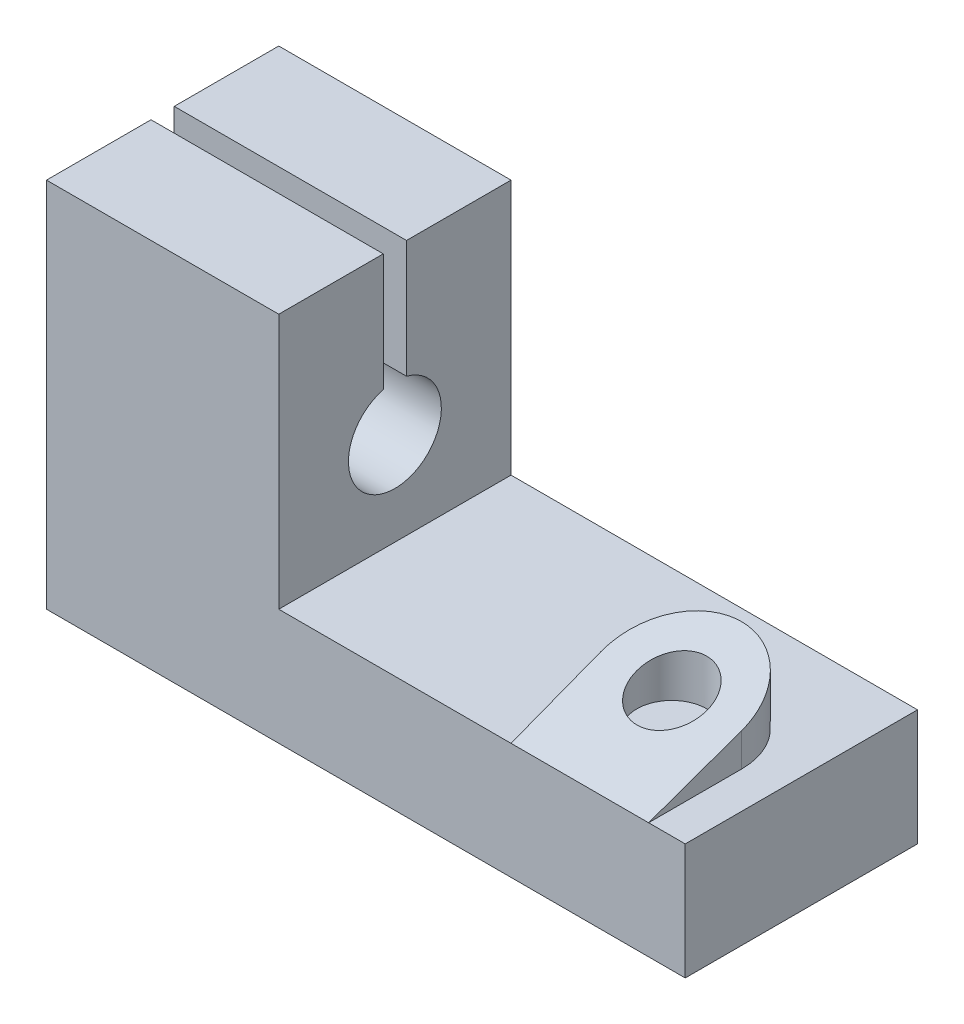
ISO-10303-21;
HEADER;
FILE_DESCRIPTION(('STEP AP214'),'2;1');
FILE_NAME('part.step','',(''),(''),'','','');
FILE_SCHEMA(('AUTOMOTIVE_DESIGN { 1 0 10303 214 1 1 1 1 }'));
ENDSEC;
DATA;
#1=APPLICATION_CONTEXT('core data for automotive mechanical design processes');
#2=APPLICATION_PROTOCOL_DEFINITION('international standard','automotive_design',2000,#1);
#3=PRODUCT_CONTEXT('',#1,'mechanical');
#4=PRODUCT('Part','Part','',(#3));
#5=PRODUCT_RELATED_PRODUCT_CATEGORY('part','',(#4));
#6=PRODUCT_DEFINITION_FORMATION('','',#4);
#7=PRODUCT_DEFINITION_CONTEXT('part definition',#1,'design');
#8=PRODUCT_DEFINITION('design','',#6,#7);
#9=PRODUCT_DEFINITION_SHAPE('','',#8);
#10=(LENGTH_UNIT() NAMED_UNIT(*) SI_UNIT(.MILLI.,.METRE.));
#11=(NAMED_UNIT(*) PLANE_ANGLE_UNIT() SI_UNIT($,.RADIAN.));
#12=(NAMED_UNIT(*) SI_UNIT($,.STERADIAN.) SOLID_ANGLE_UNIT());
#13=UNCERTAINTY_MEASURE_WITH_UNIT(LENGTH_MEASURE(1.E-05),#10,'distance_accuracy_value','');
#14=(GEOMETRIC_REPRESENTATION_CONTEXT(3) GLOBAL_UNCERTAINTY_ASSIGNED_CONTEXT((#13)) GLOBAL_UNIT_ASSIGNED_CONTEXT((#10,
#11,#12)) REPRESENTATION_CONTEXT('',''));
#15=CARTESIAN_POINT('',(0.,0.,0.));
#16=DIRECTION('',(0.,0.,1.));
#17=DIRECTION('',(1.,0.,0.));
#18=AXIS2_PLACEMENT_3D('',#15,#16,#17);
#19=CARTESIAN_POINT('',(0.,0.,20.));
#20=DIRECTION('',(1.,0.,0.));
#21=DIRECTION('',(0.,0.,-1.));
#22=AXIS2_PLACEMENT_3D('',#19,#20,#21);
#23=PLANE('',#22);
#24=DIRECTION('',(0.,1.,0.));
#25=VECTOR('',#24,1.);
#26=CARTESIAN_POINT('',(0.,0.,11.));
#27=LINE('',#26,#25);
#28=CARTESIAN_POINT('',(0.,21.8729833462074,11.));
#29=VERTEX_POINT('',#28);
#30=CARTESIAN_POINT('',(0.,32.,11.));
#31=VERTEX_POINT('',#30);
#32=EDGE_CURVE('E162',#29,#31,#27,.T.);
#33=ORIENTED_EDGE('',*,*,#32,.F.);
#34=CARTESIAN_POINT('',(0.,18.,10.));
#35=DIRECTION('',(1.,0.,0.));
#36=DIRECTION('',(0.,0.,-1.));
#37=AXIS2_PLACEMENT_3D('',#34,#35,#36);
#38=CIRCLE('',#37,4.);
#39=CARTESIAN_POINT('',(0.,21.8729833462074,9.));
#40=VERTEX_POINT('',#39);
#41=EDGE_CURVE('E176',#29,#40,#38,.T.);
#42=ORIENTED_EDGE('',*,*,#41,.T.);
#43=DIRECTION('',(0.,1.,0.));
#44=VECTOR('',#43,1.);
#45=CARTESIAN_POINT('',(0.,0.,9.));
#46=LINE('',#45,#44);
#47=CARTESIAN_POINT('',(0.,32.,9.));
#48=VERTEX_POINT('',#47);
#49=EDGE_CURVE('E64',#40,#48,#46,.T.);
#50=ORIENTED_EDGE('',*,*,#49,.T.);
#51=DIRECTION('',(0.,0.,-1.));
#52=VECTOR('',#51,1.);
#53=CARTESIAN_POINT('',(0.,32.,20.));
#54=LINE('',#53,#52);
#55=CARTESIAN_POINT('',(0.,32.,0.));
#56=VERTEX_POINT('',#55);
#57=EDGE_CURVE('E203',#48,#56,#54,.T.);
#58=ORIENTED_EDGE('',*,*,#57,.T.);
#59=DIRECTION('',(0.,-1.,0.));
#60=VECTOR('',#59,1.);
#61=CARTESIAN_POINT('',(0.,0.,0.));
#62=LINE('',#61,#60);
#63=CARTESIAN_POINT('',(0.,0.,0.));
#64=VERTEX_POINT('',#63);
#65=EDGE_CURVE('E185',#56,#64,#62,.T.);
#66=ORIENTED_EDGE('',*,*,#65,.T.);
#67=DIRECTION('',(0.,0.,-1.));
#68=VECTOR('',#67,1.);
#69=CARTESIAN_POINT('',(0.,0.,20.));
#70=LINE('',#69,#68);
#71=CARTESIAN_POINT('',(0.,0.,20.));
#72=VERTEX_POINT('',#71);
#73=EDGE_CURVE('E11',#72,#64,#70,.T.);
#74=ORIENTED_EDGE('',*,*,#73,.F.);
#75=DIRECTION('',(0.,-1.,0.));
#76=VECTOR('',#75,1.);
#77=CARTESIAN_POINT('',(0.,0.,20.));
#78=LINE('',#77,#76);
#79=CARTESIAN_POINT('',(0.,32.,20.));
#80=VERTEX_POINT('',#79);
#81=EDGE_CURVE('E183',#80,#72,#78,.T.);
#82=ORIENTED_EDGE('',*,*,#81,.F.);
#83=EDGE_CURVE('E214',#80,#31,#54,.T.);
#84=ORIENTED_EDGE('',*,*,#83,.T.);
#85=EDGE_LOOP('',(#33,#42,#50,#58,#66,#74,#82,#84));
#86=FACE_BOUND('',#85,.T.);
#87=ADVANCED_FACE('F39',(#86),#23,.F.);
#88=CARTESIAN_POINT('',(20.,32.,20.));
#89=DIRECTION('',(-1.,0.,0.));
#90=DIRECTION('',(0.,0.,1.));
#91=AXIS2_PLACEMENT_3D('',#88,#89,#90);
#92=PLANE('',#91);
#93=DIRECTION('',(0.,1.,0.));
#94=VECTOR('',#93,1.);
#95=CARTESIAN_POINT('',(20.,0.,11.));
#96=LINE('',#95,#94);
#97=CARTESIAN_POINT('',(20.,21.8729833462074,11.));
#98=VERTEX_POINT('',#97);
#99=CARTESIAN_POINT('',(20.,32.,11.));
#100=VERTEX_POINT('',#99);
#101=EDGE_CURVE('E53',#98,#100,#96,.T.);
#102=ORIENTED_EDGE('',*,*,#101,.T.);
#103=DIRECTION('',(0.,0.,-1.));
#104=VECTOR('',#103,1.);
#105=CARTESIAN_POINT('',(20.,32.,20.));
#106=LINE('',#105,#104);
#107=CARTESIAN_POINT('',(20.,32.,20.));
#108=VERTEX_POINT('',#107);
#109=EDGE_CURVE('E218',#108,#100,#106,.T.);
#110=ORIENTED_EDGE('',*,*,#109,.F.);
#111=DIRECTION('',(0.,1.,0.));
#112=VECTOR('',#111,1.);
#113=CARTESIAN_POINT('',(20.,32.,20.));
#114=LINE('',#113,#112);
#115=CARTESIAN_POINT('',(20.,10.,20.));
#116=VERTEX_POINT('',#115);
#117=EDGE_CURVE('E197',#116,#108,#114,.T.);
#118=ORIENTED_EDGE('',*,*,#117,.F.);
#119=DIRECTION('',(0.,0.,-1.));
#120=VECTOR('',#119,1.);
#121=CARTESIAN_POINT('',(20.,10.,20.));
#122=LINE('',#121,#120);
#123=CARTESIAN_POINT('',(20.,10.,0.));
#124=VERTEX_POINT('',#123);
#125=EDGE_CURVE('E225',#116,#124,#122,.T.);
#126=ORIENTED_EDGE('',*,*,#125,.T.);
#127=DIRECTION('',(0.,1.,0.));
#128=VECTOR('',#127,1.);
#129=CARTESIAN_POINT('',(20.,32.,0.));
#130=LINE('',#129,#128);
#131=CARTESIAN_POINT('',(20.,32.,0.));
#132=VERTEX_POINT('',#131);
#133=EDGE_CURVE('E209',#124,#132,#130,.T.);
#134=ORIENTED_EDGE('',*,*,#133,.T.);
#135=CARTESIAN_POINT('',(20.,32.,9.));
#136=VERTEX_POINT('',#135);
#137=EDGE_CURVE('E217',#136,#132,#106,.T.);
#138=ORIENTED_EDGE('',*,*,#137,.F.);
#139=DIRECTION('',(0.,1.,0.));
#140=VECTOR('',#139,1.);
#141=CARTESIAN_POINT('',(20.,0.,9.));
#142=LINE('',#141,#140);
#143=CARTESIAN_POINT('',(20.,21.8729833462074,9.));
#144=VERTEX_POINT('',#143);
#145=EDGE_CURVE('E164',#144,#136,#142,.T.);
#146=ORIENTED_EDGE('',*,*,#145,.F.);
#147=CARTESIAN_POINT('',(20.,18.,10.));
#148=DIRECTION('',(1.,0.,0.));
#149=DIRECTION('',(0.,0.,-1.));
#150=AXIS2_PLACEMENT_3D('',#147,#148,#149);
#151=CIRCLE('',#150,4.);
#152=EDGE_CURVE('E174',#98,#144,#151,.T.);
#153=ORIENTED_EDGE('',*,*,#152,.F.);
#154=EDGE_LOOP('',(#102,#110,#118,#126,#134,#138,#146,#153));
#155=FACE_BOUND('',#154,.T.);
#156=ADVANCED_FACE('F248',(#155),#92,.F.);
#157=CARTESIAN_POINT('',(0.,32.,20.));
#158=DIRECTION('',(0.,-1.,0.));
#159=DIRECTION('',(0.,0.,-1.));
#160=AXIS2_PLACEMENT_3D('',#157,#158,#159);
#161=PLANE('',#160);
#162=DIRECTION('',(1.,0.,0.));
#163=VECTOR('',#162,1.);
#164=CARTESIAN_POINT('',(0.,32.,11.));
#165=LINE('',#164,#163);
#166=EDGE_CURVE('E168',#31,#100,#165,.T.);
#167=ORIENTED_EDGE('',*,*,#166,.F.);
#168=ORIENTED_EDGE('',*,*,#83,.F.);
#169=DIRECTION('',(-1.,0.,0.));
#170=VECTOR('',#169,1.);
#171=CARTESIAN_POINT('',(0.,32.,20.));
#172=LINE('',#171,#170);
#173=EDGE_CURVE('E200',#108,#80,#172,.T.);
#174=ORIENTED_EDGE('',*,*,#173,.F.);
#175=ORIENTED_EDGE('',*,*,#109,.T.);
#176=EDGE_LOOP('',(#167,#168,#174,#175));
#177=FACE_BOUND('',#176,.T.);
#178=ADVANCED_FACE('F291',(#177),#161,.F.);
#179=CARTESIAN_POINT('',(0.,18.,10.));
#180=DIRECTION('',(1.,0.,0.));
#181=DIRECTION('',(0.,0.,-1.));
#182=AXIS2_PLACEMENT_3D('',#179,#180,#181);
#183=CYLINDRICAL_SURFACE('',#182,4.);
#184=DIRECTION('',(1.,0.,0.));
#185=VECTOR('',#184,1.);
#186=CARTESIAN_POINT('',(0.,21.8729833462074,11.));
#187=LINE('',#186,#185);
#188=EDGE_CURVE('E170',#29,#98,#187,.T.);
#189=ORIENTED_EDGE('',*,*,#188,.T.);
#190=ORIENTED_EDGE('',*,*,#152,.T.);
#191=DIRECTION('',(1.,0.,0.));
#192=VECTOR('',#191,1.);
#193=CARTESIAN_POINT('',(0.,21.8729833462074,9.));
#194=LINE('',#193,#192);
#195=EDGE_CURVE('E177',#40,#144,#194,.T.);
#196=ORIENTED_EDGE('',*,*,#195,.F.);
#197=ORIENTED_EDGE('',*,*,#41,.F.);
#198=EDGE_LOOP('',(#189,#190,#196,#197));
#199=FACE_BOUND('',#198,.T.);
#200=ADVANCED_FACE('F296',(#199),#183,.F.);
#201=CARTESIAN_POINT('',(0.,0.,20.));
#202=DIRECTION('',(0.,1.,0.));
#203=DIRECTION('',(0.,0.,1.));
#204=AXIS2_PLACEMENT_3D('',#201,#202,#203);
#205=PLANE('',#204);
#206=DIRECTION('',(1.,0.,0.));
#207=VECTOR('',#206,1.);
#208=CARTESIAN_POINT('',(0.,0.,0.));
#209=LINE('',#208,#207);
#210=CARTESIAN_POINT('',(55.,0.,0.));
#211=VERTEX_POINT('',#210);
#212=EDGE_CURVE('E204',#64,#211,#209,.T.);
#213=ORIENTED_EDGE('',*,*,#212,.T.);
#214=DIRECTION('',(0.,0.,-1.));
#215=VECTOR('',#214,1.);
#216=CARTESIAN_POINT('',(55.,0.,20.));
#217=LINE('',#216,#215);
#218=CARTESIAN_POINT('',(55.,0.,20.));
#219=VERTEX_POINT('',#218);
#220=EDGE_CURVE('E50',#219,#211,#217,.T.);
#221=ORIENTED_EDGE('',*,*,#220,.F.);
#222=DIRECTION('',(1.,0.,0.));
#223=VECTOR('',#222,1.);
#224=CARTESIAN_POINT('',(0.,0.,20.));
#225=LINE('',#224,#223);
#226=EDGE_CURVE('E190',#72,#219,#225,.T.);
#227=ORIENTED_EDGE('',*,*,#226,.F.);
#228=ORIENTED_EDGE('',*,*,#73,.T.);
#229=EDGE_LOOP('',(#213,#221,#227,#228));
#230=FACE_BOUND('',#229,.T.);
#231=ADVANCED_FACE('F308',(#230),#205,.F.);
#232=CARTESIAN_POINT('',(55.,0.,20.));
#233=DIRECTION('',(-1.,0.,0.));
#234=DIRECTION('',(0.,0.,1.));
#235=AXIS2_PLACEMENT_3D('',#232,#233,#234);
#236=PLANE('',#235);
#237=DIRECTION('',(0.,1.,0.));
#238=VECTOR('',#237,1.);
#239=CARTESIAN_POINT('',(55.,0.,0.));
#240=LINE('',#239,#238);
#241=CARTESIAN_POINT('',(55.,10.,0.));
#242=VERTEX_POINT('',#241);
#243=EDGE_CURVE('E206',#211,#242,#240,.T.);
#244=ORIENTED_EDGE('',*,*,#243,.T.);
#245=DIRECTION('',(0.,0.,-1.));
#246=VECTOR('',#245,1.);
#247=CARTESIAN_POINT('',(55.,10.,20.));
#248=LINE('',#247,#246);
#249=CARTESIAN_POINT('',(55.,10.,20.));
#250=VERTEX_POINT('',#249);
#251=EDGE_CURVE('E223',#250,#242,#248,.T.);
#252=ORIENTED_EDGE('',*,*,#251,.F.);
#253=DIRECTION('',(0.,1.,0.));
#254=VECTOR('',#253,1.);
#255=CARTESIAN_POINT('',(55.,0.,20.));
#256=LINE('',#255,#254);
#257=EDGE_CURVE('E192',#219,#250,#256,.T.);
#258=ORIENTED_EDGE('',*,*,#257,.F.);
#259=ORIENTED_EDGE('',*,*,#220,.T.);
#260=EDGE_LOOP('',(#244,#252,#258,#259));
#261=FACE_BOUND('',#260,.T.);
#262=ADVANCED_FACE('F235',(#261),#236,.F.);
#263=CARTESIAN_POINT('',(20.,10.,20.));
#264=DIRECTION('',(0.,-1.,0.));
#265=DIRECTION('',(0.,0.,-1.));
#266=AXIS2_PLACEMENT_3D('',#263,#264,#265);
#267=PLANE('',#266);
#268=DIRECTION('',(0.0193826635216767,0.,0.999812138531437));
#269=VECTOR('',#268,1.);
#270=CARTESIAN_POINT('',(39.8471641057222,10.,12.1162959811301));
#271=LINE('',#270,#269);
#272=CARTESIAN_POINT('',(39.8471641057222,10.,12.1162959811301));
#273=VERTEX_POINT('',#272);
#274=CARTESIAN_POINT('',(40.,10.,20.));
#275=VERTEX_POINT('',#274);
#276=EDGE_CURVE('E157',#273,#275,#271,.T.);
#277=ORIENTED_EDGE('',*,*,#276,.F.);
#278=CARTESIAN_POINT('',(45.8460369369108,10.,12.));
#279=DIRECTION('',(0.,1.,0.));
#280=DIRECTION('',(0.,0.,1.));
#281=AXIS2_PLACEMENT_3D('',#278,#279,#280);
#282=CIRCLE('',#281,6.);
#283=CARTESIAN_POINT('',(51.8460369369108,10.,12.));
#284=VERTEX_POINT('',#283);
#285=EDGE_CURVE('E256',#284,#273,#282,.T.);
#286=ORIENTED_EDGE('',*,*,#285,.F.);
#287=DIRECTION('',(0.,0.,-1.));
#288=VECTOR('',#287,1.);
#289=CARTESIAN_POINT('',(51.8460369369108,10.,20.));
#290=LINE('',#289,#288);
#291=CARTESIAN_POINT('',(51.8460369369108,10.,20.));
#292=VERTEX_POINT('',#291);
#293=EDGE_CURVE('E154',#292,#284,#290,.T.);
#294=ORIENTED_EDGE('',*,*,#293,.F.);
#295=DIRECTION('',(-1.,0.,0.));
#296=VECTOR('',#295,1.);
#297=CARTESIAN_POINT('',(20.,10.,20.));
#298=LINE('',#297,#296);
#299=EDGE_CURVE('E191',#250,#292,#298,.T.);
#300=ORIENTED_EDGE('',*,*,#299,.F.);
#301=ORIENTED_EDGE('',*,*,#251,.T.);
#302=DIRECTION('',(-1.,0.,0.));
#303=VECTOR('',#302,1.);
#304=CARTESIAN_POINT('',(20.,10.,0.));
#305=LINE('',#304,#303);
#306=EDGE_CURVE('E208',#242,#124,#305,.T.);
#307=ORIENTED_EDGE('',*,*,#306,.T.);
#308=ORIENTED_EDGE('',*,*,#125,.F.);
#309=EDGE_CURVE('E195',#275,#116,#298,.T.);
#310=ORIENTED_EDGE('',*,*,#309,.F.);
#311=EDGE_LOOP('',(#277,#286,#294,#300,#301,#307,#308,#310));
#312=FACE_BOUND('',#311,.T.);
#313=ADVANCED_FACE('F243',(#312),#267,.F.);
#314=ORIENTED_EDGE('',*,*,#57,.F.);
#315=DIRECTION('',(1.,0.,0.));
#316=VECTOR('',#315,1.);
#317=CARTESIAN_POINT('',(0.,32.,9.));
#318=LINE('',#317,#316);
#319=EDGE_CURVE('E175',#48,#136,#318,.T.);
#320=ORIENTED_EDGE('',*,*,#319,.T.);
#321=ORIENTED_EDGE('',*,*,#137,.T.);
#322=DIRECTION('',(-1.,0.,0.));
#323=VECTOR('',#322,1.);
#324=CARTESIAN_POINT('',(0.,32.,0.));
#325=LINE('',#324,#323);
#326=EDGE_CURVE('E186',#132,#56,#325,.T.);
#327=ORIENTED_EDGE('',*,*,#326,.T.);
#328=EDGE_LOOP('',(#314,#320,#321,#327));
#329=FACE_BOUND('',#328,.T.);
#330=ADVANCED_FACE('F287',(#329),#161,.F.);
#331=CARTESIAN_POINT('',(0.,0.,20.));
#332=DIRECTION('',(0.,0.,-1.));
#333=DIRECTION('',(-1.,0.,0.));
#334=AXIS2_PLACEMENT_3D('',#331,#332,#333);
#335=PLANE('',#334);
#336=ORIENTED_EDGE('',*,*,#299,.T.);
#337=DIRECTION('',(1.,0.,0.));
#338=VECTOR('',#337,1.);
#339=CARTESIAN_POINT('',(39.8460369369108,10.,20.));
#340=LINE('',#339,#338);
#341=EDGE_CURVE('E147',#275,#292,#340,.T.);
#342=ORIENTED_EDGE('',*,*,#341,.F.);
#343=ORIENTED_EDGE('',*,*,#309,.T.);
#344=ORIENTED_EDGE('',*,*,#117,.T.);
#345=ORIENTED_EDGE('',*,*,#173,.T.);
#346=ORIENTED_EDGE('',*,*,#81,.T.);
#347=ORIENTED_EDGE('',*,*,#226,.T.);
#348=ORIENTED_EDGE('',*,*,#257,.T.);
#349=EDGE_LOOP('',(#336,#342,#343,#344,#345,#346,#347,#348));
#350=FACE_BOUND('',#349,.T.);
#351=ADVANCED_FACE('F254',(#350),#335,.F.);
#352=CARTESIAN_POINT('',(0.,0.,0.));
#353=DIRECTION('',(0.,0.,-1.));
#354=DIRECTION('',(-1.,0.,0.));
#355=AXIS2_PLACEMENT_3D('',#352,#353,#354);
#356=PLANE('',#355);
#357=ORIENTED_EDGE('',*,*,#65,.F.);
#358=ORIENTED_EDGE('',*,*,#326,.F.);
#359=ORIENTED_EDGE('',*,*,#133,.F.);
#360=ORIENTED_EDGE('',*,*,#306,.F.);
#361=ORIENTED_EDGE('',*,*,#243,.F.);
#362=ORIENTED_EDGE('',*,*,#212,.F.);
#363=EDGE_LOOP('',(#357,#358,#359,#360,#361,#362));
#364=FACE_BOUND('',#363,.T.);
#365=ADVANCED_FACE('F239',(#364),#356,.T.);
#366=CARTESIAN_POINT('',(0.,0.,9.));
#367=DIRECTION('',(0.,0.,-1.));
#368=DIRECTION('',(-1.,0.,0.));
#369=AXIS2_PLACEMENT_3D('',#366,#367,#368);
#370=PLANE('',#369);
#371=ORIENTED_EDGE('',*,*,#145,.T.);
#372=ORIENTED_EDGE('',*,*,#319,.F.);
#373=ORIENTED_EDGE('',*,*,#49,.F.);
#374=ORIENTED_EDGE('',*,*,#195,.T.);
#375=EDGE_LOOP('',(#371,#372,#373,#374));
#376=FACE_BOUND('',#375,.T.);
#377=ADVANCED_FACE('F304',(#376),#370,.F.);
#378=CARTESIAN_POINT('',(0.,0.,11.));
#379=DIRECTION('',(0.,0.,-1.));
#380=DIRECTION('',(-1.,0.,0.));
#381=AXIS2_PLACEMENT_3D('',#378,#379,#380);
#382=PLANE('',#381);
#383=ORIENTED_EDGE('',*,*,#101,.F.);
#384=ORIENTED_EDGE('',*,*,#188,.F.);
#385=ORIENTED_EDGE('',*,*,#32,.T.);
#386=ORIENTED_EDGE('',*,*,#166,.T.);
#387=EDGE_LOOP('',(#383,#384,#385,#386));
#388=FACE_BOUND('',#387,.T.);
#389=ADVANCED_FACE('F321',(#388),#382,.T.);
#390=CARTESIAN_POINT('',(45.8460369369108,15.,12.));
#391=DIRECTION('',(0.,-1.,0.));
#392=DIRECTION('',(0.,0.,-1.));
#393=AXIS2_PLACEMENT_3D('',#390,#391,#392);
#394=CYLINDRICAL_SURFACE('',#393,6.);
#395=DIRECTION('',(0.,-1.,0.));
#396=VECTOR('',#395,1.);
#397=CARTESIAN_POINT('',(39.8471641057222,15.,12.1162959811301));
#398=LINE('',#397,#396);
#399=CARTESIAN_POINT('',(39.8471641057222,12.8156085781678,12.1162959811301));
#400=VERTEX_POINT('',#399);
#401=EDGE_CURVE('E138',#400,#273,#398,.T.);
#402=ORIENTED_EDGE('',*,*,#401,.F.);
#403=CARTESIAN_POINT('',(45.8460369369108,12.8571428571429,12.));
#404=DIRECTION('',(0.,-0.941741911594837,-0.336336396998156));
#405=DIRECTION('',(0.,-0.336336396998156,0.941741911594838));
#406=AXIS2_PLACEMENT_3D('',#403,#404,#405);
#407=ELLIPSE('',#406,6.37117232027936,6.);
#408=CARTESIAN_POINT('',(51.8460369369108,12.8571428571429,12.));
#409=VERTEX_POINT('',#408);
#410=EDGE_CURVE('E135',#400,#409,#407,.T.);
#411=ORIENTED_EDGE('',*,*,#410,.T.);
#412=DIRECTION('',(0.,-1.,0.));
#413=VECTOR('',#412,1.);
#414=CARTESIAN_POINT('',(51.8460369369108,15.,12.));
#415=LINE('',#414,#413);
#416=EDGE_CURVE('E140',#409,#284,#415,.T.);
#417=ORIENTED_EDGE('',*,*,#416,.T.);
#418=ORIENTED_EDGE('',*,*,#285,.T.);
#419=EDGE_LOOP('',(#402,#411,#417,#418));
#420=FACE_BOUND('',#419,.T.);
#421=ADVANCED_FACE('F133',(#420),#394,.T.);
#422=CARTESIAN_POINT('',(39.8471641057222,15.,12.1162959811301));
#423=DIRECTION('',(0.999812138531437,0.,-0.0193826635216767));
#424=DIRECTION('',(-0.0193826635216767,0.,-0.999812138531437));
#425=AXIS2_PLACEMENT_3D('',#422,#423,#424);
#426=PLANE('',#425);
#427=ORIENTED_EDGE('',*,*,#276,.T.);
#428=DIRECTION('',(-0.0182538544824765,0.336280358147225,-0.94158500281223));
#429=VECTOR('',#428,1.);
#430=CARTESIAN_POINT('',(39.8337554096266,13.0626293446399,11.4246378350084));
#431=LINE('',#430,#429);
#432=EDGE_CURVE('E145',#275,#400,#431,.T.);
#433=ORIENTED_EDGE('',*,*,#432,.T.);
#434=ORIENTED_EDGE('',*,*,#401,.T.);
#435=EDGE_LOOP('',(#427,#433,#434));
#436=FACE_BOUND('',#435,.T.);
#437=ADVANCED_FACE('F361',(#436),#426,.F.);
#438=CARTESIAN_POINT('',(51.8460369369108,15.,20.));
#439=DIRECTION('',(-1.,0.,0.));
#440=DIRECTION('',(0.,0.,1.));
#441=AXIS2_PLACEMENT_3D('',#438,#439,#440);
#442=PLANE('',#441);
#443=ORIENTED_EDGE('',*,*,#416,.F.);
#444=DIRECTION('',(0.,0.336336396998156,-0.941741911594837));
#445=VECTOR('',#444,1.);
#446=CARTESIAN_POINT('',(51.8460369369108,15.,6.));
#447=LINE('',#446,#445);
#448=EDGE_CURVE('E150',#292,#409,#447,.T.);
#449=ORIENTED_EDGE('',*,*,#448,.F.);
#450=ORIENTED_EDGE('',*,*,#293,.T.);
#451=EDGE_LOOP('',(#443,#449,#450));
#452=FACE_BOUND('',#451,.T.);
#453=ADVANCED_FACE('F152',(#452),#442,.F.);
#454=CARTESIAN_POINT('',(39.8460369369108,15.,6.));
#455=DIRECTION('',(0.,-0.941741911594837,-0.336336396998156));
#456=DIRECTION('',(0.,0.336336396998156,-0.941741911594838));
#457=AXIS2_PLACEMENT_3D('',#454,#455,#456);
#458=PLANE('',#457);
#459=CARTESIAN_POINT('',(45.8460369369108,12.8571428571429,12.));
#460=DIRECTION('',(0.,-0.941741911594837,-0.336336396998156));
#461=DIRECTION('',(0.,-0.336336396998156,0.941741911594838));
#462=AXIS2_PLACEMENT_3D('',#459,#460,#461);
#463=ELLIPSE('',#462,3.18558616013968,3.);
#464=CARTESIAN_POINT('',(45.8460369369108,11.7857142857143,15.));
#465=VERTEX_POINT('',#464);
#466=EDGE_CURVE('E45',#465,#465,#463,.T.);
#467=ORIENTED_EDGE('',*,*,#466,.T.);
#468=EDGE_LOOP('',(#467));
#469=FACE_BOUND('',#468,.T.);
#470=ORIENTED_EDGE('',*,*,#410,.F.);
#471=ORIENTED_EDGE('',*,*,#432,.F.);
#472=ORIENTED_EDGE('',*,*,#341,.T.);
#473=ORIENTED_EDGE('',*,*,#448,.T.);
#474=EDGE_LOOP('',(#470,#471,#472,#473));
#475=FACE_BOUND('',#474,.T.);
#476=ADVANCED_FACE('F146',(#469,#475),#458,.F.);
#477=CARTESIAN_POINT('',(45.8460369369108,10.,12.));
#478=DIRECTION('',(0.,1.,0.));
#479=DIRECTION('',(0.,0.,1.));
#480=AXIS2_PLACEMENT_3D('',#477,#478,#479);
#481=CIRCLE('',#480,3.);
#482=CARTESIAN_POINT('',(45.8460369369108,10.,15.));
#483=VERTEX_POINT('',#482);
#484=EDGE_CURVE('E141',#483,#483,#481,.T.);
#485=ORIENTED_EDGE('',*,*,#484,.T.);
#486=EDGE_LOOP('',(#485));
#487=FACE_BOUND('',#486,.T.);
#488=ADVANCED_FACE('F275',(#487),#267,.F.);
#489=CARTESIAN_POINT('',(45.8460369369108,15.,12.));
#490=DIRECTION('',(0.,-1.,0.));
#491=DIRECTION('',(0.,0.,-1.));
#492=AXIS2_PLACEMENT_3D('',#489,#490,#491);
#493=CYLINDRICAL_SURFACE('',#492,3.);
#494=ORIENTED_EDGE('',*,*,#466,.F.);
#495=EDGE_LOOP('',(#494));
#496=FACE_BOUND('',#495,.T.);
#497=ORIENTED_EDGE('',*,*,#484,.F.);
#498=EDGE_LOOP('',(#497));
#499=FACE_BOUND('',#498,.T.);
#500=ADVANCED_FACE('F267',(#496,#499),#493,.F.);
#501=CLOSED_SHELL('',(#87,#156,#178,#200,#231,#262,#313,#330,#351,#365,#377,#389,#421,#437,#453,
#476,#488,#500));
#502=MANIFOLD_SOLID_BREP('B2',#501);
#503=ADVANCED_BREP_SHAPE_REPRESENTATION('',(#18,#502),#14);
#504=SHAPE_DEFINITION_REPRESENTATION(#9,#503);
ENDSEC;
END-ISO-10303-21;
